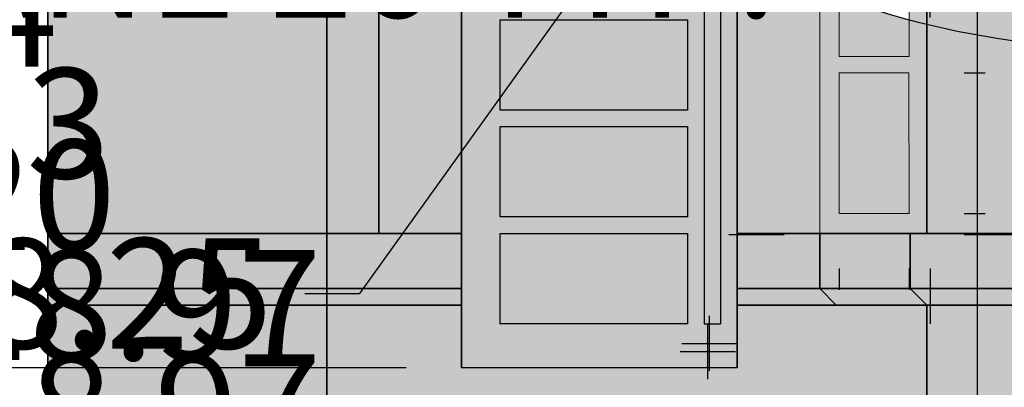
# Model space of a CAD drawing. Units: millimetres. Extents: x 130 to 1021, y 147 to 699.
# Tile 3 of 40: x 302 to 481, y 246 to 313. Entities that reach past the tile are written whole.
import ezdxf

# ---------------------------------------------------------------- set-up
doc = ezdxf.new("R2010")
doc.units = ezdxf.units.MM
doc.header["$MEASUREMENT"] = 0
for name, color, linetype, lineweight in [('A-ANNO-DIMS', 2, 'Continuous', 18), ('A-DOOR', 3, 'Continuous', 25), ('A-ELEV', 7, 'Continuous', 35), ('A-ELEV-PATT', 9, 'Continuous', 13), ('A-FLOR-STRS', 2, 'Continuous', 25), ('A-GLAZ', 4, 'Continuous', 18)]:
    doc.layers.add(name, color=color, linetype=linetype, lineweight=lineweight)
doc.styles.get("Standard").update_dxf_attribs({"font": 'arial.ttf'})
doc.dimstyles.get("Standard").update_dxf_attribs({"dimtxt": 20, "dimasz": 10, "dimexe": 10, "dimexo": 10, "dimgap": 5, "dimtad": 0, "dimtih": 1, "dimtoh": 1, "dimdec": 0, "dimzin": 0, "dimdsep": 46, "dimtxsty": 'Standard', "dimcen": 5, "dimadec": 0, "dimazin": 0, "dimtfac": 1, "dimtdec": 0, "dimtofl": 0, "dimtmove": 0, "dimatfit": 3, "dimfxl": 1, "dimtolj": 1, "dimtzin": 0, "dimarcsym": 0})

# ---------------------------------------------------------------- blocks, each defined once
blk = doc.blocks.new('DOOR-PANEL')
for p, q in [((0, 16.4), (34, 16.4)), ((0, 0), (0, 16.4)), ((34, 16.4), (34, 0)), ((34, 0), (0, 0))]:
    blk.add_line(p, q)
blk = doc.blocks.new('WIN-SIDELIGHT-PANE')
for p, q in [((0, 25.55), (12.68, 25.55)), ((0, 0), (0, 25.55)), ((12.68, 25.55), (12.68, 0)), ((12.68, 0), (0, 0))]:
    blk.add_line(p, q)
blk = doc.blocks.new('*D7')
at = {"layer": 'A-ANNO-DIMS', "color": 0, "lineweight": -2, "transparency": 16777216}
for p, q in [((399.37, 349.45), (413.37, 349.45)), ((423.37, 349.45), (433.37, 349.45)), ((389.37, 344.55), (389.37, 339.45)), ((423.37, 344.55), (423.37, 339.45))]:
    blk.add_line(p, q, dxfattribs=at)
at = {"layer": 'A-ANNO-DIMS', "color": 0, "transparency": 16777216}
for points in [[(399.37, 351.11), (399.37, 347.78), (389.37, 349.45)], [(413.37, 351.11), (413.37, 347.78), (423.37, 349.45)]]:
    blk.add_solid(points, dxfattribs=at)
at = {"layer": 'Defpoints', "color": 0, "transparency": 16777216}
for p in [(389.37, 354.55), (423.37, 354.55), (423.37, 349.45)]:
    blk.add_point(p, dxfattribs=at)
at = {"layer": 'A-ANNO-DIMS', "color": 0, "transparency": 16777216, "insert": (582.04, 349.45), "char_height": 20, "attachment_point": 5}
blk.add_mtext('\\A1;DOOR PANEL 34 TYP.', dxfattribs=at)
blk = doc.blocks.new('*D9')
at = {"layer": 'A-ANNO-DIMS', "color": 0, "lineweight": -2, "transparency": 16777216}
for p, q in [((467.37, 323.13), (457.37, 323.13)), ((467.37, 313.13), (467.37, 323.13)), ((473.55, 303.13), (477.38, 303.13)), ((473.57, 277.58), (477.4, 277.58)), ((467.41, 267.57), (467.42, 257.57))]:
    blk.add_line(p, q, dxfattribs=at)
at = {"layer": 'A-ANNO-DIMS', "color": 0, "transparency": 16777216}
for points in [[(469.04, 313.13), (465.71, 313.13), (467.38, 303.13)], [(469.08, 267.57), (465.75, 267.57), (467.4, 277.57)]]:
    blk.add_solid(points, dxfattribs=at)
at = {"layer": 'Defpoints', "color": 0, "transparency": 16777216}
for p in [(463.55, 303.12), (467.38, 303.13), (463.57, 277.57)]:
    blk.add_point(p, dxfattribs=at)
at = {"layer": 'A-ANNO-DIMS', "color": 0, "transparency": 16777216, "insert": (284.19, 323.13), "char_height": 20, "attachment_point": 5}
blk.add_mtext('\\A1;SIDELIGHT PANE 26 TYP.', dxfattribs=at)
blk = doc.blocks.new('*D10')
at = {"layer": 'A-ANNO-DIMS', "color": 0, "lineweight": -2, "transparency": 16777216}
for p, q in [((440.89, 273.72), (430.89, 273.71)), ((473.57, 273.75), (483.57, 273.75)), ((450.9, 267.56), (450.9, 263.73)), ((463.58, 267.57), (463.58, 263.74))]:
    blk.add_line(p, q, dxfattribs=at)
at = {"layer": 'A-ANNO-DIMS', "color": 0, "transparency": 16777216}
for points in [[(440.89, 275.38), (440.89, 272.05), (450.89, 273.73)], [(473.57, 275.41), (473.58, 272.08), (463.57, 273.74)]]:
    blk.add_solid(points, dxfattribs=at)
at = {"layer": 'Defpoints', "color": 0, "transparency": 16777216}
for p in [(450.89, 277.56), (463.57, 277.57), (463.57, 273.74)]:
    blk.add_point(p, dxfattribs=at)
at = {"layer": 'A-ANNO-DIMS', "color": 0, "transparency": 16777216, "insert": (536.31, 273.75), "char_height": 20, "attachment_point": 5}
blk.add_mtext('\\A1;13 TYP.', dxfattribs=at)
blk = doc.blocks.new('*D11')
at = {"layer": 'A-ANNO-DIMS', "color": 0, "lineweight": -2, "transparency": 16777216}
for p, q in [((737.37, 648.7), (737.37, 149.74)), ((299.37, 566.95), (299.37, 149.74)), ((309.37, 159.74), (490.86, 159.74)), ((727.37, 159.74), (545.89, 159.74))]:
    blk.add_line(p, q, dxfattribs=at)
at = {"layer": 'A-ANNO-DIMS', "color": 0, "transparency": 16777216}
for points in [[(309.37, 161.41), (309.37, 158.07), (299.37, 159.74)], [(727.37, 161.41), (727.37, 158.07), (737.37, 159.74)]]:
    blk.add_solid(points, dxfattribs=at)
at = {"layer": 'Defpoints', "color": 0, "transparency": 16777216}
for p in [(737.37, 658.7), (299.37, 576.95), (737.37, 159.74)]:
    blk.add_point(p, dxfattribs=at)
at = {"layer": 'A-ANNO-DIMS', "color": 0, "transparency": 16777216, "insert": (518.37, 159.74), "char_height": 20, "attachment_point": 5}
blk.add_mtext('\\A1;438', dxfattribs=at)
blk = doc.blocks.new('*D12')
at = {"layer": 'A-ANNO-DIMS', "color": 0, "lineweight": -2, "transparency": 16777216}
for p, q in [((477.37, 661.95), (265.07, 661.95)), ((275.07, 651.95), (275.07, 438.2)), ((275.07, 194.04), (275.07, 407.78)), ((357.16, 184.04), (265.07, 184.04))]:
    blk.add_line(p, q, dxfattribs=at)
at = {"layer": 'A-ANNO-DIMS', "color": 0, "transparency": 16777216}
for points in [[(273.41, 651.95), (276.74, 651.95), (275.07, 661.95)], [(273.41, 194.04), (276.74, 194.04), (275.07, 184.04)]]:
    blk.add_solid(points, dxfattribs=at)
at = {"layer": 'Defpoints', "color": 0, "transparency": 16777216}
for p in [(275.07, 661.95), (487.37, 661.95), (367.16, 184.04)]:
    blk.add_point(p, dxfattribs=at)
at = {"layer": 'A-ANNO-DIMS', "color": 0, "transparency": 16777216, "insert": (275.07, 422.99), "char_height": 20, "attachment_point": 5}
blk.add_mtext('\\A1;477.9', dxfattribs=at)
blk = doc.blocks.new('*D23')
at = {"layer": 'A-ANNO-DIMS', "color": 0, "lineweight": -2, "transparency": 16777216}
for p, q in [((466.77, 403.95), (466.77, 696.25)), ((475.99, 209.04), (475.99, 696.25)), ((456.77, 686.25), (446.77, 686.25)), ((485.99, 686.25), (495.99, 686.25))]:
    blk.add_line(p, q, dxfattribs=at)
at = {"layer": 'A-ANNO-DIMS', "color": 0, "transparency": 16777216}
for points in [[(456.77, 687.91), (456.77, 684.58), (466.77, 686.25)], [(485.99, 687.91), (485.99, 684.58), (475.99, 686.25)]]:
    blk.add_solid(points, dxfattribs=at)
at = {"layer": 'Defpoints', "color": 0, "transparency": 16777216}
for p in [(475.99, 686.25), (466.77, 393.95), (475.99, 199.04)]:
    blk.add_point(p, dxfattribs=at)
at = {"layer": 'A-ANNO-DIMS', "color": 0, "transparency": 16777216, "insert": (534.63, 686.25), "char_height": 20, "attachment_point": 5}
blk.add_mtext('\\A1;9.222', dxfattribs=at)
blk = doc.blocks.new('*D24')
at = {"layer": 'A-ANNO-DIMS', "color": 0, "lineweight": -2, "transparency": 16777216}
for p, q in [((475.99, 209.04), (475.99, 696.25)), ((487.37, 671.95), (487.37, 696.25)), ((465.99, 686.25), (455.99, 686.25)), ((497.37, 686.25), (507.37, 686.25))]:
    blk.add_line(p, q, dxfattribs=at)
at = {"layer": 'A-ANNO-DIMS', "color": 0, "transparency": 16777216}
for points in [[(465.99, 687.91), (465.99, 684.58), (475.99, 686.25)], [(497.37, 687.91), (497.37, 684.58), (487.37, 686.25)]]:
    blk.add_solid(points, dxfattribs=at)
at = {"layer": 'Defpoints', "color": 0, "transparency": 16777216}
for p in [(487.37, 686.25), (487.37, 661.95), (475.99, 199.04)]:
    blk.add_point(p, dxfattribs=at)
at = {"layer": 'A-ANNO-DIMS', "color": 0, "transparency": 16777216, "insert": (553.02, 686.25), "char_height": 20, "attachment_point": 5}
blk.add_mtext('\\A1;11.385', dxfattribs=at)
blk = doc.blocks.new('*D34')
at = {"layer": 'A-ANNO-DIMS', "color": 0, "lineweight": -2, "transparency": 16777216}
for p, q in [((275.07, 231.98), (275.07, 241.98)), ((275.07, 241.98), (285.07, 241.98)), ((459.84, 221.98), (265.07, 221.98)), ((462.91, 203.01), (265.07, 203.01)), ((275.07, 193.01), (275.07, 183.01))]:
    blk.add_line(p, q, dxfattribs=at)
at = {"layer": 'A-ANNO-DIMS', "color": 0, "transparency": 16777216}
for points in [[(273.41, 231.98), (276.74, 231.98), (275.07, 221.98)], [(273.41, 193.01), (276.74, 193.01), (275.07, 203.01)]]:
    blk.add_solid(points, dxfattribs=at)
at = {"layer": 'Defpoints', "color": 0, "transparency": 16777216}
for p in [(275.07, 221.98), (469.84, 221.98), (472.91, 203.01)]:
    blk.add_point(p, dxfattribs=at)
at = {"layer": 'A-ANNO-DIMS', "color": 0, "transparency": 16777216, "insert": (322.88, 241.98), "char_height": 20, "attachment_point": 5}
blk.add_mtext('\\A1;18.97', dxfattribs=at)
blk = doc.blocks.new('*D35')
at = {"layer": 'A-ANNO-DIMS', "color": 0, "lineweight": -2, "transparency": 16777216}
for p, q in [((275.07, 250.95), (275.07, 260.95)), ((275.07, 260.95), (285.07, 260.95)), ((456.77, 240.95), (265.07, 240.95)), ((459.84, 221.98), (265.07, 221.98)), ((275.07, 211.98), (275.07, 201.98))]:
    blk.add_line(p, q, dxfattribs=at)
at = {"layer": 'A-ANNO-DIMS', "color": 0, "transparency": 16777216}
for points in [[(273.41, 250.95), (276.74, 250.95), (275.07, 240.95)], [(273.41, 211.98), (276.74, 211.98), (275.07, 221.98)]]:
    blk.add_solid(points, dxfattribs=at)
at = {"layer": 'Defpoints', "color": 0, "transparency": 16777216}
for p in [(275.07, 240.95), (466.77, 240.95), (469.84, 221.98)]:
    blk.add_point(p, dxfattribs=at)
at = {"layer": 'A-ANNO-DIMS', "color": 0, "transparency": 16777216, "insert": (322.88, 260.95), "char_height": 20, "attachment_point": 5}
blk.add_mtext('\\A1;18.97', dxfattribs=at)
blk = doc.blocks.new('*D36')
at = {"layer": 'A-ANNO-DIMS', "color": 0, "lineweight": -2, "transparency": 16777216}
for p, q in [((275.07, 270.95), (275.07, 280.95)), ((275.07, 280.95), (285.07, 280.95)), ((297.37, 260.95), (265.07, 260.95)), ((456.77, 240.95), (265.07, 240.95)), ((275.07, 230.95), (275.07, 220.95))]:
    blk.add_line(p, q, dxfattribs=at)
at = {"layer": 'A-ANNO-DIMS', "color": 0, "transparency": 16777216}
for points in [[(273.41, 270.95), (276.74, 270.95), (275.07, 260.95)], [(273.41, 230.95), (276.74, 230.95), (275.07, 240.95)]]:
    blk.add_solid(points, dxfattribs=at)
at = {"layer": 'Defpoints', "color": 0, "transparency": 16777216}
for p in [(275.07, 260.95), (307.37, 260.95), (466.77, 240.95)]:
    blk.add_point(p, dxfattribs=at)
at = {"layer": 'A-ANNO-DIMS', "color": 0, "transparency": 16777216, "insert": (304.53, 280.95), "char_height": 20, "attachment_point": 5}
blk.add_mtext('\\A1;20', dxfattribs=at)
blk = doc.blocks.new('*D37')
at = {"layer": 'A-ANNO-DIMS', "color": 0, "lineweight": -2, "transparency": 16777216}
for p, q in [((275.07, 283.95), (275.07, 293.95)), ((275.07, 293.95), (285.07, 293.95)), ((297.37, 273.95), (265.07, 273.95)), ((297.37, 260.95), (265.07, 260.95)), ((275.07, 250.95), (275.07, 240.95))]:
    blk.add_line(p, q, dxfattribs=at)
at = {"layer": 'A-ANNO-DIMS', "color": 0, "transparency": 16777216}
for points in [[(273.41, 283.95), (276.74, 283.95), (275.07, 273.95)], [(273.41, 250.95), (276.74, 250.95), (275.07, 260.95)]]:
    blk.add_solid(points, dxfattribs=at)
at = {"layer": 'Defpoints', "color": 0, "transparency": 16777216}
for p in [(275.07, 273.95), (307.37, 273.95), (307.37, 260.95)]:
    blk.add_point(p, dxfattribs=at)
at = {"layer": 'A-ANNO-DIMS', "color": 0, "transparency": 16777216, "insert": (303.46, 293.95), "char_height": 20, "attachment_point": 5}
blk.add_mtext('\\A1;13', dxfattribs=at)
blk = doc.blocks.new('*D38')
at = {"layer": 'A-ANNO-DIMS', "color": 0, "lineweight": -2, "transparency": 16777216}
for p, q in [((297.37, 388.95), (265.07, 388.95)), ((275.07, 378.95), (275.07, 346.66)), ((275.07, 283.95), (275.07, 316.24)), ((297.37, 273.95), (265.07, 273.95))]:
    blk.add_line(p, q, dxfattribs=at)
at = {"layer": 'A-ANNO-DIMS', "color": 0, "transparency": 16777216}
for points in [[(273.41, 378.95), (276.74, 378.95), (275.07, 388.95)], [(273.41, 283.95), (276.74, 283.95), (275.07, 273.95)]]:
    blk.add_solid(points, dxfattribs=at)
at = {"layer": 'Defpoints', "color": 0, "transparency": 16777216}
for p in [(275.07, 388.95), (307.37, 388.95), (307.37, 273.95)]:
    blk.add_point(p, dxfattribs=at)
at = {"layer": 'A-ANNO-DIMS', "color": 0, "transparency": 16777216, "insert": (275.07, 331.45), "char_height": 20, "attachment_point": 5}
blk.add_mtext('\\A1;115', dxfattribs=at)
blk = doc.blocks.new('*D60')
at = {"layer": 'A-ANNO-DIMS', "color": 0, "lineweight": -2, "transparency": 16777216}
for p, q in [((372.37, 378.95), (265.07, 378.95)), ((275.07, 368.95), (275.07, 329.46)), ((275.07, 259.55), (275.07, 299.04)), ((372.37, 249.55), (265.07, 249.55))]:
    blk.add_line(p, q, dxfattribs=at)
at = {"layer": 'A-ANNO-DIMS', "color": 0, "transparency": 16777216}
for points in [[(273.41, 368.95), (276.74, 368.95), (275.07, 378.95)], [(273.41, 259.55), (276.74, 259.55), (275.07, 249.55)]]:
    blk.add_solid(points, dxfattribs=at)
at = {"layer": 'Defpoints', "color": 0, "transparency": 16777216}
for p in [(275.07, 378.95), (382.37, 378.95), (382.37, 249.55)]:
    blk.add_point(p, dxfattribs=at)
at = {"layer": 'A-ANNO-DIMS', "color": 0, "transparency": 16777216, "insert": (275.07, 314.25), "char_height": 20, "attachment_point": 5}
blk.add_mtext('\\A1;129.4', dxfattribs=at)
blk = doc.blocks.new('*D64')
at = {"layer": 'A-ANNO-DIMS', "color": 0, "lineweight": -2, "transparency": 16777216}
for p, q in [((502.05, 450.93), (502.05, 460.93)), ((497.05, 455.93), (507.05, 455.93)), ((363.96, 263.06), (409.92, 327.25)), ((353.96, 263.06), (363.96, 263.06))]:
    blk.add_line(p, q, dxfattribs=at)
at = {"layer": 'A-ANNO-DIMS', "color": 0, "transparency": 16777216}
blk.add_solid([(408.57, 328.22), (411.28, 326.28), (415.74, 335.39)], dxfattribs=at)
at = {"layer": 'Defpoints', "color": 0, "transparency": 16777216}
for p in [(502.05, 455.93), (415.74, 335.39)]:
    blk.add_point(p, dxfattribs=at)
at = {"layer": 'A-ANNO-DIMS', "color": 0, "transparency": 16777216, "insert": (297.8, 263.06), "char_height": 20, "attachment_point": 5}
blk.add_mtext('\\A1;R148.25', dxfattribs=at)
blk = doc.blocks.new('*D65')
at = {"layer": 'A-ANNO-DIMS', "color": 0, "lineweight": -2, "transparency": 16777216}
for p, q in [((495.46, 509.13), (472.51, 423.11)), ((505.46, 509.13), (495.46, 509.13)), ((427.37, 248.98), (427.37, 258.98)), ((422.37, 253.98), (432.37, 253.98))]:
    blk.add_line(p, q, dxfattribs=at)
at = {"layer": 'A-ANNO-DIMS', "color": 0, "transparency": 16777216}
blk.add_solid([(470.9, 423.54), (474.12, 422.68), (469.93, 413.45)], dxfattribs=at)
at = {"layer": 'Defpoints', "color": 0, "transparency": 16777216}
for p in [(469.93, 413.45), (427.37, 253.98)]:
    blk.add_point(p, dxfattribs=at)
at = {"layer": 'A-ANNO-DIMS', "color": 0, "transparency": 16777216, "insert": (561.62, 509.13), "char_height": 20, "attachment_point": 5}
blk.add_mtext('\\A1;R165.05', dxfattribs=at)
blk = doc.blocks.new('*D67')
at = {"layer": 'A-ANNO-DIMS', "color": 0, "lineweight": -2, "transparency": 16777216}
for p, q in [((479.76, 492.43), (462.14, 412.22)), ((489.76, 492.43), (479.76, 492.43)), ((427.07, 247.5), (427.07, 257.5)), ((422.07, 252.5), (432.07, 252.5))]:
    blk.add_line(p, q, dxfattribs=at)
at = {"layer": 'A-ANNO-DIMS', "color": 0, "transparency": 16777216}
blk.add_solid([(460.52, 412.58), (463.77, 411.87), (460, 402.46)], dxfattribs=at)
at = {"layer": 'Defpoints', "color": 0, "transparency": 16777216}
for p in [(460, 402.46), (427.07, 252.5)]:
    blk.add_point(p, dxfattribs=at)
at = {"layer": 'A-ANNO-DIMS', "color": 0, "transparency": 16777216, "insert": (545.84, 492.43), "char_height": 20, "attachment_point": 5}
blk.add_mtext('\\A1;R153.53', dxfattribs=at)

msp = doc.modelspace()

# ---------------------------------------------------------------- hatches: boundary and pattern name
at = {"layer": 'A-ELEV-PATT'}
h = msp.add_hatch(color=256, dxfattribs=at)
h.dxf.hatch_style = 1
h.paths.add_polyline_path([(737.3738, 658.6988, 0.01359606), (632.4019, 661.9473), (607.3738, 661.9473), (487.3738, 661.9473), (487.3738, 649.9473), (607.3738, 649.9473), (632.3794, 649.9473, -0.01368411), (737.3738, 646.6784)])
h.paths.add_polyline_path([(732.3738, 643.9599, 0.01305286), (632.3738, 646.9473), (607.3738, 646.9473), (487.3738, 646.9473), (487.3738, 596.9473), (632.3738, 596.9473, -0.01305286), (732.3738, 593.9599)])
h.paths.add_polyline_path([(737.3738, 593.6732, 0.01370629), (632.3738, 596.9473), (487.3738, 596.9473), (487.3738, 586.9473), (632.355, 586.9473, -0.01378075), (737.3738, 583.6559)])
h.paths.add_polyline_path([(447.3738, 646.9473), (307.3738, 646.9473), (302.3738, 646.9473), (302.3738, 634.9473), (447.3738, 634.9473)])
h.paths.add_polyline_path([(447.3738, 631.9473), (307.3738, 631.9473), (307.3738, 586.9473), (447.3738, 586.9473)])
h.paths.add_polyline_path([(447.3738, 586.9473), (307.3738, 586.9473), (302.3738, 586.9473), (302.3738, 576.9473), (447.3738, 576.9473)])
h.paths.add_polyline_path([(447.3738, 573.9473), (367.3738, 573.9473), (367.3738, 539.9473), (447.3738, 539.9473)])
h.paths.add_polyline_path([(447.3738, 537.9473), (367.3738, 537.9473), (367.3738, 507.9473), (400.392, 507.4253, -0.00172798), (401.3281, 507.6451, -0.52200255), (425.6117, 511.0391, -0.03918489), (447.3738, 510.4359), (447.3738, 510.7883)])
h.paths.add_polyline_path([(394.7238, 505.9473), (367.3738, 505.9473), (367.3738, 476.9473, -0.0146512), (375.8501, 480.2159), (376.1506, 499.2266, -0.03554194)])
h.paths.add_polyline_path([(632.3738, 583.9473), (552.3738, 583.9473), (552.3738, 550.9473), (632.3738, 550.9473)])
h.paths.add_polyline_path([(632.3738, 548.9473), (552.3738, 548.9473), (552.3738, 515.9473), (632.3738, 515.9473)])
h.paths.add_polyline_path([(632.3738, 513.9473), (552.3738, 513.9473), (552.3738, 476.9473), (632.3738, 476.9473)])
h.paths.add_polyline_path([(737.3738, 473.6903, 0.01363261), (632.3926, 476.9473), (552.3738, 476.9473), (487.3738, 476.9473), (487.3738, 466.9473), (632.3738, 466.9473, -0.01370629), (737.3738, 463.6732)])
h.paths.add_polyline_path([(732.3738, 460.9552, 0.01307409), (632.3681, 463.9473), (487.3738, 463.9473), (487.3738, 407.735, -0.00322862), (489.3544, 406.9473), (632.3926, 406.9473, -0.01298259), (732.3738, 403.9755)])
h.paths.add_polyline_path([(487.3738, 463.9473, 0.20132998), (367.3738, 463.9473), (367.3738, 407.735, -0.18820307), (487.3738, 407.735)])
h.paths.add_polyline_path([(367.3738, 476.9473), (367.3738, 466.9473, -0.20133085), (487.3738, 466.9473), (487.3738, 476.9473, 0.20132998)])
h.paths.add_polyline_path([(367.3738, 463.9473), (307.3738, 463.9473), (307.3738, 401.9473), (357.9413, 401.9473), (367.3738, 407.735)])
h.paths.add_polyline_path([(367.3738, 476.9473), (302.3738, 476.9473), (302.3738, 466.9473), (367.3738, 466.9473)])
h.paths.add_polyline_path([(632.8184, 366.9453), (552.3738, 366.9453), (552.3738, 393.9473), (632.8184, 393.9473)])
h.paths.add_polyline_path([(632.8184, 357.2114), (632.8184, 363.9453), (552.3738, 363.9453), (552.3738, 357.2114), (552.3738, 336.9453), (632.8184, 336.9453)])
h.paths.add_polyline_path([(632.8184, 333.9453), (552.3738, 333.9453), (552.3738, 306.9453), (632.8184, 306.9453)])
h.paths.add_polyline_path([(632.8184, 303.9453), (552.3738, 303.9453), (552.3738, 273.9473), (632.355, 273.9473, 0.00006077), (632.8184, 273.9491)])
h.paths.add_polyline_path([(737.3738, 403.6903, 0.01363261), (632.3926, 406.9473), (489.3544, 406.9473, 0.19154808), (367.3738, 407.735), (367.3738, 396.9473, -0.20133085), (487.3738, 396.9473), (632.3738, 396.9473, -0.01370629), (737.3738, 393.6732)])
h.paths.add_polyline_path([(357.9413, 401.9473), (307.3738, 401.9473), (307.3738, 391.9473), (357.9413, 391.9473)])
h.paths.add_polyline_path([(357.9413, 357.2114), (357.9413, 388.9473), (307.3738, 388.9473), (307.3738, 357.2114), (307.3738, 273.9473), (357.9413, 273.9473)])
h.paths.add_polyline_path([(732.3738, 263.93, -0.0130317), (632.3794, 260.9473), (466.7667, 260.9473), (466.7667, 240.9473), (469.8406, 236.978), (469.8406, 221.978), (472.9145, 218.0087), (472.9145, 213.9473), (607.3738, 213.9473), (732.3738, 213.9473)])
h.paths.add_polyline_path([(732.3738, 290.889), (722.479, 290.889), (722.479, 301.889), (732.3738, 301.889), (732.3738, 305.889), (722.479, 305.889), (722.479, 316.889), (732.3738, 316.889), (732.3738, 320.889), (722.479, 320.889), (722.479, 331.889), (732.3738, 331.889), (732.3738, 335.889), (722.479, 335.889), (722.479, 346.889), (732.3738, 346.889), (732.3738, 350.889), (722.479, 350.889), (722.479, 361.889), (732.3738, 361.889), (732.3738, 365.889), (722.479, 365.889), (722.479, 376.889), (732.3738, 376.889), (732.3738, 380.889), (722.479, 380.889), (722.479, 391.4848, 0.00052326), (718.479, 391.6843), (718.479, 380.889), (707.479, 380.889), (707.479, 392.1896, 0.00052307), (703.479, 392.3576), (703.479, 380.889), (692.479, 380.889), (692.479, 392.7765, 0.00052292), (688.479, 392.9131), (688.479, 380.889), (677.479, 380.889), (677.479, 393.2456, 0.00052279), (673.479, 393.3508), (673.479, 380.889), (662.479, 380.889), (662.479, 393.597, 0.0005227), (658.479, 393.6709), (658.479, 380.889), (647.479, 380.889), (647.479, 393.8308, 0.00052264), (643.479, 393.8732), (643.479, 380.889), (632.8184, 380.889), (632.8184, 376.889), (643.479, 376.889), (643.479, 365.889), (632.8184, 365.889), (632.8184, 361.889), (643.479, 361.889), (643.479, 350.889), (632.8184, 350.889), (632.8184, 346.889), (643.479, 346.889), (643.479, 335.889), (632.8184, 335.889), (632.8184, 331.889), (643.479, 331.889), (643.479, 320.889), (632.8184, 320.889), (632.8184, 316.889), (643.479, 316.889), (643.479, 305.889), (632.8184, 305.889), (632.8184, 301.889), (643.479, 301.889), (643.479, 290.889), (632.8184, 290.889), (632.8184, 286.889), (643.479, 286.889), (643.479, 274.0217, 0.00052456), (647.479, 274.0643), (647.479, 286.889), (658.479, 286.889), (658.479, 274.2248, 0.00052462), (662.479, 274.2989), (662.479, 286.889), (673.479, 286.889), (673.479, 274.546, 0.00052471), (677.479, 274.6516), (677.479, 286.889), (688.479, 286.889), (688.479, 274.9853, 0.00052484), (692.479, 275.1224), (692.479, 286.889), (703.479, 286.889), (703.479, 275.5429, 0.000525), (707.479, 275.7115), (707.479, 286.889), (718.479, 286.889), (718.479, 276.2187, 0.00052519), (722.479, 276.4189), (722.479, 286.889), (732.3738, 286.889)])
h.paths.add_polyline_path([(718.479, 290.889), (707.479, 290.889), (707.479, 301.889), (718.479, 301.889)], flags=16)
h.paths.add_polyline_path([(703.479, 290.889), (692.479, 290.889), (692.479, 301.889), (703.479, 301.889)], flags=16)
h.paths.add_polyline_path([(718.479, 305.889), (707.479, 305.889), (707.479, 316.889), (718.479, 316.889)], flags=16)
h.paths.add_polyline_path([(703.479, 305.889), (692.479, 305.889), (692.479, 316.889), (703.479, 316.889)], flags=16)
h.paths.add_polyline_path([(688.479, 290.889), (677.479, 290.889), (677.479, 301.889), (688.479, 301.889)], flags=16)
h.paths.add_polyline_path([(718.479, 320.889), (707.479, 320.889), (707.479, 331.889), (718.479, 331.889)], flags=16)
h.paths.add_polyline_path([(688.479, 305.889), (677.479, 305.889), (677.479, 316.889), (688.479, 316.889)], flags=16)
h.paths.add_polyline_path([(703.479, 320.889), (692.479, 320.889), (692.479, 331.889), (703.479, 331.889)], flags=16)
h.paths.add_polyline_path([(688.479, 320.889), (677.479, 320.889), (677.479, 331.889), (688.479, 331.889)], flags=16)
h.paths.add_polyline_path([(673.479, 290.889), (662.479, 290.889), (662.479, 301.889), (673.479, 301.889)], flags=16)
h.paths.add_polyline_path([(718.479, 335.889), (707.479, 335.889), (707.479, 346.889), (718.479, 346.889)], flags=16)
h.paths.add_polyline_path([(673.479, 305.889), (662.479, 305.889), (662.479, 316.889), (673.479, 316.889)], flags=16)
h.paths.add_polyline_path([(703.479, 335.889), (692.479, 335.889), (692.479, 346.889), (703.479, 346.889)], flags=16)
h.paths.add_polyline_path([(673.479, 320.889), (662.479, 320.889), (662.479, 331.889), (673.479, 331.889)], flags=16)
h.paths.add_polyline_path([(688.479, 335.889), (677.479, 335.889), (677.479, 346.889), (688.479, 346.889)], flags=16)
h.paths.add_polyline_path([(658.479, 290.889), (647.479, 290.889), (647.479, 301.889), (658.479, 301.889)], flags=16)
h.paths.add_polyline_path([(718.479, 350.889), (707.479, 350.889), (707.479, 361.889), (718.479, 361.889)], flags=16)
h.paths.add_polyline_path([(658.479, 305.889), (647.479, 305.889), (647.479, 316.889), (658.479, 316.889)], flags=16)
h.paths.add_polyline_path([(703.479, 350.889), (692.479, 350.889), (692.479, 361.889), (703.479, 361.889)], flags=16)
h.paths.add_polyline_path([(673.479, 335.889), (662.479, 335.889), (662.479, 346.889), (673.479, 346.889)], flags=16)
h.paths.add_polyline_path([(658.479, 320.889), (647.479, 320.889), (647.479, 331.889), (658.479, 331.889)], flags=16)
h.paths.add_polyline_path([(688.479, 350.889), (677.479, 350.889), (677.479, 361.889), (688.479, 361.889)], flags=16)
h.paths.add_polyline_path([(718.479, 365.889), (707.479, 365.889), (707.479, 376.889), (718.479, 376.889)], flags=16)
h.paths.add_polyline_path([(658.479, 335.889), (647.479, 335.889), (647.479, 346.889), (658.479, 346.889)], flags=16)
h.paths.add_polyline_path([(673.479, 350.889), (662.479, 350.889), (662.479, 361.889), (673.479, 361.889)], flags=16)
h.paths.add_polyline_path([(703.479, 365.889), (692.479, 365.889), (692.479, 376.889), (703.479, 376.889)], flags=16)
h.paths.add_polyline_path([(688.479, 365.889), (677.479, 365.889), (677.479, 376.889), (688.479, 376.889)], flags=16)
h.paths.add_polyline_path([(658.479, 350.889), (647.479, 350.889), (647.479, 361.889), (658.479, 361.889)], flags=16)
h.paths.add_polyline_path([(673.479, 365.889), (662.479, 365.889), (662.479, 376.889), (673.479, 376.889)], flags=16)
h.paths.add_polyline_path([(658.479, 365.889), (647.479, 365.889), (647.479, 376.889), (658.479, 376.889)], flags=16)
h.paths.add_polyline_path([(732.3738, 503.9786), (722.3392, 503.9786), (722.3392, 514.9786), (732.3738, 514.9786), (732.3738, 518.9786), (722.3392, 518.9786), (722.3392, 529.9786), (732.3738, 529.9786), (732.3738, 533.9786), (722.3392, 533.9786), (722.3392, 544.9786), (732.3738, 544.9786), (732.3738, 546.9473), (732.3738, 548.9786), (722.3392, 548.9786), (722.3392, 559.9786), (732.3738, 559.9786), (732.3738, 563.9786), (722.3392, 563.9786), (722.3392, 574.9786), (732.3738, 574.9786), (732.3738, 578.9786), (722.3392, 578.9786), (722.3392, 581.4789, 0.00052601), (718.3392, 581.6791), (718.3392, 578.9786), (707.3392, 578.9786), (707.3392, 582.1863, 0.00052582), (703.3392, 582.355), (703.3392, 578.9786), (692.3392, 578.9786), (692.3392, 582.7752, 0.00052566), (688.3392, 582.9123), (688.3392, 578.9786), (677.3392, 578.9786), (677.3392, 583.2457, 0.00052554), (673.3392, 583.3512), (673.3392, 578.9786), (662.3392, 578.9786), (662.3392, 583.5978, 0.00052545), (658.3392, 583.6718), (658.3392, 578.9786), (647.3392, 578.9786), (647.3392, 583.8317, 0.00052539), (643.3392, 583.8741), (643.3392, 578.9786), (632.3738, 578.9786), (632.3738, 574.9786), (643.3392, 574.9786), (643.3392, 563.9786), (632.3738, 563.9786), (632.3738, 559.9786), (643.3392, 559.9786), (643.3392, 548.9786), (632.3738, 548.9786), (632.3738, 544.9786), (643.3392, 544.9786), (643.3392, 533.9786), (632.3738, 533.9786), (632.3738, 529.9786), (643.3392, 529.9786), (643.3392, 518.9786), (632.3738, 518.9786), (632.3738, 515.9473), (632.3738, 514.9786), (643.3392, 514.9786), (643.3392, 503.9786), (632.3738, 503.9786), (632.3738, 499.9786), (643.3392, 499.9786), (643.3392, 488.9786), (632.3738, 488.9786), (632.3738, 484.9786), (643.3392, 484.9786), (643.3392, 476.8751, -0.00051911), (647.3392, 476.8332), (647.3392, 484.9786), (658.3392, 484.9786), (658.3392, 476.6752, -0.00051917), (662.3392, 476.6022), (662.3392, 484.9786), (673.3392, 484.9786), (673.3392, 476.3585, -0.00051926), (677.3392, 476.2543), (677.3392, 484.9786), (688.3392, 484.9786), (688.3392, 475.9248, -0.00051938), (692.3392, 475.7894), (692.3392, 484.9786), (703.3392, 484.9786), (703.3392, 475.3741, -0.00051953), (707.3392, 475.2075), (707.3392, 484.9786), (718.3392, 484.9786), (718.3392, 474.7064, -0.00051972), (722.3392, 474.5086), (722.3392, 484.9786), (732.3738, 484.9786), (732.3738, 488.9786), (722.3392, 488.9786), (722.3392, 499.9786), (732.3738, 499.9786)])
h.paths.add_polyline_path([(718.3392, 503.9786), (707.3392, 503.9786), (707.3392, 514.9786), (718.3392, 514.9786)], flags=16)
h.paths.add_polyline_path([(718.3392, 499.9786), (718.3392, 488.9786), (707.3392, 488.9786), (707.3392, 499.9786)], flags=16)
h.paths.add_polyline_path([(718.3392, 518.9786), (707.3392, 518.9786), (707.3392, 529.9786), (718.3392, 529.9786)], flags=16)
h.paths.add_polyline_path([(703.3392, 503.9786), (692.3392, 503.9786), (692.3392, 514.9786), (703.3392, 514.9786)], flags=16)
h.paths.add_polyline_path([(703.3392, 499.9786), (703.3392, 488.9786), (692.3392, 488.9786), (692.3392, 499.9786)], flags=16)
h.paths.add_polyline_path([(703.3392, 518.9786), (692.3392, 518.9786), (692.3392, 529.9786), (703.3392, 529.9786)], flags=16)
h.paths.add_polyline_path([(718.3392, 533.9786), (707.3392, 533.9786), (707.3392, 544.9786), (718.3392, 544.9786)], flags=16)
h.paths.add_polyline_path([(688.3392, 503.9786), (677.3392, 503.9786), (677.3392, 514.9786), (688.3392, 514.9786)], flags=16)
h.paths.add_polyline_path([(688.3392, 499.9786), (688.3392, 488.9786), (677.3392, 488.9786), (677.3392, 499.9786)], flags=16)
h.paths.add_polyline_path([(703.3392, 533.9786), (692.3392, 533.9786), (692.3392, 544.9786), (703.3392, 544.9786)], flags=16)
h.paths.add_polyline_path([(688.3392, 518.9786), (677.3392, 518.9786), (677.3392, 529.9786), (688.3392, 529.9786)], flags=16)
h.paths.add_polyline_path([(688.3392, 533.9786), (677.3392, 533.9786), (677.3392, 544.9786), (688.3392, 544.9786)], flags=16)
h.paths.add_polyline_path([(718.3392, 548.9786), (707.3392, 548.9786), (707.3392, 559.9786), (718.3392, 559.9786)], flags=16)
h.paths.add_polyline_path([(673.3392, 503.9786), (662.3392, 503.9786), (662.3392, 514.9786), (673.3392, 514.9786)], flags=16)
h.paths.add_polyline_path([(673.3392, 499.9786), (673.3392, 488.9786), (662.3392, 488.9786), (662.3392, 499.9786)], flags=16)
h.paths.add_polyline_path([(703.3392, 548.9786), (692.3392, 548.9786), (692.3392, 559.9786), (703.3392, 559.9786)], flags=16)
h.paths.add_polyline_path([(673.3392, 518.9786), (662.3392, 518.9786), (662.3392, 529.9786), (673.3392, 529.9786)], flags=16)
h.paths.add_polyline_path([(688.3392, 548.9786), (677.3392, 548.9786), (677.3392, 559.9786), (688.3392, 559.9786)], flags=16)
h.paths.add_polyline_path([(673.3392, 533.9786), (662.3392, 533.9786), (662.3392, 544.9786), (673.3392, 544.9786)], flags=16)
h.paths.add_polyline_path([(718.3392, 563.9786), (707.3392, 563.9786), (707.3392, 574.9786), (718.3392, 574.9786)], flags=16)
h.paths.add_polyline_path([(658.3392, 503.9786), (647.3392, 503.9786), (647.3392, 514.9786), (658.3392, 514.9786)], flags=16)
h.paths.add_polyline_path([(658.3392, 499.9786), (658.3392, 488.9786), (647.3392, 488.9786), (647.3392, 499.9786)], flags=16)
h.paths.add_polyline_path([(703.3392, 563.9786), (692.3392, 563.9786), (692.3392, 574.9786), (703.3392, 574.9786)], flags=16)
h.paths.add_polyline_path([(658.3392, 518.9786), (647.3392, 518.9786), (647.3392, 529.9786), (658.3392, 529.9786)], flags=16)
h.paths.add_polyline_path([(673.3392, 548.9786), (662.3392, 548.9786), (662.3392, 559.9786), (673.3392, 559.9786)], flags=16)
h.paths.add_polyline_path([(688.3392, 563.9786), (677.3392, 563.9786), (677.3392, 574.9786), (688.3392, 574.9786)], flags=16)
h.paths.add_polyline_path([(658.3392, 533.9786), (647.3392, 533.9786), (647.3392, 544.9786), (658.3392, 544.9786)], flags=16)
h.paths.add_polyline_path([(673.3392, 563.9786), (662.3392, 563.9786), (662.3392, 574.9786), (673.3392, 574.9786)], flags=16)
h.paths.add_polyline_path([(658.3392, 548.9786), (647.3392, 548.9786), (647.3392, 559.9786), (658.3392, 559.9786)], flags=16)
h.paths.add_polyline_path([(658.3392, 563.9786), (647.3392, 563.9786), (647.3392, 574.9786), (658.3392, 574.9786)], flags=16)
h = msp.add_hatch(color=256, dxfattribs=at)
h.dxf.hatch_style = 1
h.paths.add_polyline_path([(447.3738, 576.9473), (302.3738, 576.9473), (302.3738, 573.9473), (447.3738, 573.9473)])
h.paths.add_polyline_path([(487.3738, 583.9473), (487.3738, 586.9473), (447.3738, 576.9473), (447.3738, 573.9473)])
h.paths.add_polyline_path([(632.355, 586.9473), (487.3738, 586.9473), (487.3738, 583.9473), (632.3738, 583.9473), (632.3738, 583.9472, -0.01380003), (737.3738, 580.6507), (737.3738, 583.6559, 0.01378075)])
h.paths.add_polyline_path([(367.3738, 466.9473), (302.3738, 466.9473), (302.3738, 463.9473), (367.3738, 463.9473)])
h.paths.add_polyline_path([(487.3738, 463.9473), (487.3738, 466.9473, 0.20133085), (367.3738, 466.9473), (367.3738, 463.9473, -0.20132998)])
h.paths.add_polyline_path([(632.3738, 466.9473), (487.3738, 466.9473), (487.3738, 463.9473), (632.3681, 463.9473, -0.01372855), (737.3738, 460.6681), (737.3738, 463.6732, 0.01370629)])
h.paths.add_polyline_path([(632.3738, 396.9473), (487.3738, 396.9473, 0.20133085), (367.3738, 396.9473), (367.3738, 393.9473, -0.20237172), (486.7667, 393.9473), (632.3681, 393.9473, -0.01372855), (737.3738, 390.6681), (737.3738, 393.6732, 0.01370629)])
h.paths.add_polyline_path([(357.9413, 391.9473), (307.3738, 391.9473), (307.3738, 388.9473), (357.9413, 388.9473)])
h.paths.add_polyline_path([(367.3738, 393.9473), (367.3738, 396.9473), (357.9413, 391.924), (357.9413, 388.9473), (358.058, 388.9473)])
h.paths.add_polyline_path([(737.3738, 264.2162), (737.3738, 267.2214, -0.01370629), (632.3738, 263.9473), (463.7667, 263.9473), (466.7667, 260.9473), (632.3794, 260.9473, 0.01368411)])
h.paths.add_polyline_path([(463.7667, 263.9473), (447.3738, 263.9473), (450.3738, 260.9473), (466.7667, 260.9473)])
h.paths.add_polyline_path([(447.3738, 263.9473), (432.3738, 263.9473), (432.3738, 260.9473), (450.3738, 260.9473)])
h.paths.add_polyline_path([(382.3738, 263.9473), (357.9413, 263.9473), (357.9413, 260.9473), (382.3738, 260.9473)])
h.paths.add_polyline_path([(357.9413, 263.9473), (307.3738, 263.9473), (307.3738, 260.9473), (357.9413, 260.9473)])
h = msp.add_hatch(color=256, dxfattribs=at)
h.paths.add_polyline_path([(327.3738, 569.884), (327.3738, 573.9473), (307.3738, 573.9473), (307.3738, 476.9473), (327.3738, 476.9473), (327.3738, 480.95)])
h.paths.add_polyline_path([(486.7667, 386.2639), (486.7667, 393.9473), (466.7667, 393.9473), (466.7667, 357.2114), (466.7667, 311.9335, 0.03427026), (486.7667, 308.4637)])
h.paths.add_polyline_path([(486.7667, 308.4637, -0.03427026), (466.7667, 311.9335), (466.7667, 273.9473), (486.7667, 273.9473)])
h.paths.add_polyline_path([(389.3738, 351.5473), (396.7693, 351.5473, -0.00702703), (393.8774, 354.5473), (389.3738, 354.5473), (389.3738, 359.5775, -0.01903024), (382.3738, 368.424), (382.3738, 249.5473), (432.3738, 249.5473), (432.3738, 325.067, -0.00576734), (429.3738, 326.709), (429.3738, 257.5473), (426.3738, 257.5473), (426.3738, 328.4428, -0.00592542), (423.3738, 330.272), (423.3738, 315.7473), (389.3738, 315.7473), (389.3738, 332.1473), (420.4552, 332.1473, -0.00895099), (416.0768, 335.1473), (389.3738, 335.1473)])
h.paths.add_polyline_path([(389.3738, 312.7473), (423.3738, 312.7473), (423.3738, 296.3473), (389.3738, 296.3473)], flags=16)
h.paths.add_polyline_path([(389.3738, 293.3473), (423.3738, 293.3473), (423.3738, 276.9473), (389.3738, 276.9473)], flags=16)
h.paths.add_polyline_path([(389.3738, 273.9473), (423.3738, 273.9473), (423.3738, 257.5473), (389.3738, 257.5473)], flags=16)
h.paths.add_polyline_path([(432.3738, 378.9473), (382.3738, 378.9473), (382.3738, 368.424, 0.01903024), (389.3738, 359.5775), (389.3738, 370.9473), (423.3738, 370.9473), (423.3738, 354.5473), (393.8774, 354.5473, 0.00702703), (396.7693, 351.5473), (423.3738, 351.5473), (423.3738, 335.1473), (416.0768, 335.1473, 0.00895099), (420.4552, 332.1473), (423.3738, 332.1473), (423.3738, 330.272, 0.00592542), (426.3738, 328.4428), (426.3738, 370.9473), (429.3738, 370.9473), (429.3738, 326.709, 0.00576734), (432.3738, 325.067)])
h.paths.add_polyline_path([(466.7667, 357.2114), (466.7667, 393.9473), (447.3738, 393.9473), (447.3738, 357.2114), (447.3738, 318.1243, 0.0063261), (450.8779, 316.785), (450.8779, 331.5915), (463.5608, 331.5915), (463.5608, 312.7571, 0.00558197), (466.7667, 311.9335)])
h.paths.add_polyline_path([(450.8779, 334.5915), (450.8779, 360.0915), (463.5608, 360.0915), (463.5608, 334.5915)], flags=16)
h.paths.add_polyline_path([(450.8779, 363.0915), (450.8779, 388.6449), (463.5608, 388.6449), (463.5608, 363.0915)], flags=16)
h.paths.add_polyline_path([(466.7667, 311.9335, -0.00558197), (463.5608, 312.7571), (463.5608, 306.0915), (450.8779, 306.0915), (450.8779, 316.785, -0.0063261), (447.3738, 318.1243), (447.3738, 273.9473), (466.7667, 273.9473)])
h.paths.add_polyline_path([(450.8779, 303.0915), (463.5608, 303.0915), (463.5608, 277.5915), (450.8779, 277.5915)], flags=16)
h.paths.add_polyline_path([(552.3738, 357.2114), (552.3738, 393.9473), (486.7667, 393.9473), (486.7667, 386.2639), (544.6354, 386.2639), (544.6354, 280.6619), (486.7667, 280.6619), (486.7667, 273.9473), (552.3738, 273.9473)])
h.paths.add_polyline_path([(487.3738, 583.9473), (472.3738, 580.1973), (472.3738, 507.0765), (472.3738, 505.4251, -0.00564525), (475.3738, 504.4942), (475.3738, 506.3543), (475.3738, 511.9473), (484.3738, 511.9473), (484.3738, 503.8134), (484.3738, 501.2439, -0.00583574), (487.3738, 500.0015)])
h.paths.add_polyline_path([(484.3738, 578.0434), (484.3738, 548.9473), (475.3738, 548.9473), (475.3738, 575.7934)], flags=16)
h.paths.add_polyline_path([(484.3738, 546.9473), (484.3738, 513.9473), (475.3738, 513.9473), (475.3738, 518.7148), (475.3738, 546.9473)], flags=16)
h = msp.add_hatch(color=256, dxfattribs=at)
h.dxf.hatch_style = 1
h.paths.add_polyline_path([(367.3738, 407.735), (357.9413, 401.9473), (357.9413, 391.9473), (357.985, 391.9473), (367.3738, 396.9473)])
h.paths.add_polyline_path([(367.3738, 393.9473), (357.9413, 388.8847), (357.9413, 357.2114), (357.9413, 273.9473), (367.3738, 273.9473), (367.3738, 357.2114)])
h = msp.add_hatch(color=256, dxfattribs=at)
h.dxf.hatch_style = 1
h.paths.add_polyline_path([(382.3738, 368.424, -0.05004781), (367.3738, 393.9473), (367.3738, 357.2114), (367.3738, 273.9473), (382.3738, 273.9473)])
h.paths.add_polyline_path([(432.3738, 273.9473), (447.3738, 273.9473), (447.3738, 318.1243, -0.02789446), (432.3738, 325.067)])
h.paths.add_polyline_path([(463.5608, 306.0915), (463.5608, 312.7571, -0.02245133), (450.8779, 316.785), (450.8779, 306.0915)])
h.paths.add_polyline_path([(450.8779, 303.0915), (450.8779, 277.5915), (463.5608, 277.5915), (463.5608, 303.0915)])
h = msp.add_hatch(color=256, dxfattribs=at)
h.set_gradient(color1=(221, 197, 207), color2=(86, 84, 89), name='CURVED')
h.paths.add_polyline_path([(423.3738, 273.9473), (389.3738, 273.9473), (389.3738, 257.5473), (423.3738, 257.5473)])
h.paths.add_polyline_path([(423.3738, 293.3473), (389.3738, 293.3473), (389.3738, 276.9473), (423.3738, 276.9473)])
h.paths.add_polyline_path([(423.3738, 312.7473), (389.3738, 312.7473), (389.3738, 296.3473), (423.3738, 296.3473)])
h.paths.add_polyline_path([(423.3738, 330.272, -0.00585023), (420.4552, 332.1473), (389.3738, 332.1473), (389.3738, 315.7473), (423.3738, 315.7473)])
h.paths.add_polyline_path([(396.7693, 351.5473), (389.3738, 351.5473), (389.3738, 335.1473), (416.0768, 335.1473, -0.04279691)])
h.paths.add_polyline_path([(423.3738, 351.5473), (396.7693, 351.5473, 0.04279691), (416.0768, 335.1473), (423.3738, 335.1473)])
h.paths.add_polyline_path([(423.3738, 370.9473), (389.3738, 370.9473), (389.3738, 359.5775, 0.01138691), (393.8774, 354.5473), (423.3738, 354.5473)])
h.paths.add_polyline_path([(389.3738, 359.5775), (389.3738, 354.5473), (393.8774, 354.5473, -0.01138691)], flags=17)
h = msp.add_hatch(color=256, dxfattribs=at)
h.set_gradient(color1=(221, 197, 207), color2=(86, 84, 89), name='CURVED')
h.paths.add_polyline_path([(429.3738, 326.709, -0.00584318), (426.3738, 328.4428), (426.3738, 257.5473), (429.3738, 257.5473)])
h.paths.add_polyline_path([(426.3738, 328.4428, 0.00584318), (429.3738, 326.709), (429.3738, 370.9473), (426.3738, 370.9473)])
h = msp.add_hatch(color=256, dxfattribs=at)
h.dxf.hatch_style = 1
h.paths.add_polyline_path([(463.7667, 273.9473), (463.7667, 263.9473), (632.3738, 263.9473, 0.01370629), (737.3738, 267.2214), (737.3738, 277.2387, -0.01378075), (632.355, 273.9473)])
h = msp.add_hatch(color=256, dxfattribs=at)
h.dxf.hatch_style = 1
h.paths.add_polyline_path([(357.9413, 240.9473), (357.9413, 260.9473), (307.3738, 260.9473), (307.3738, 213.9473), (357.9413, 213.9473)])
h.paths.add_polyline_path([(382.3738, 260.9473), (357.9413, 260.9473), (357.9413, 240.9473), (466.7667, 240.9473), (466.7667, 260.9473), (432.3738, 260.9473), (432.3738, 249.5473), (382.3738, 249.5473)])
h.paths.add_polyline_path([(357.9413, 273.9473), (307.3738, 273.9473), (307.3738, 263.9473), (357.9413, 263.9473)])
h.paths.add_polyline_path([(382.3738, 273.9473), (357.9413, 273.9473), (357.9413, 263.9473), (382.3738, 263.9473)])
msp.add_hatch(color=256, dxfattribs=at).paths.add_polyline_path([(432.3738, 273.9473), (432.3738, 263.9473), (447.3738, 263.9473), (447.3738, 273.9473)])
h = msp.add_hatch(color=256, dxfattribs=at)
h.set_gradient(color1=(199, 200, 202), color2=(147, 149, 152), name='HEMISPHERICAL')
h.paths.add_polyline_path([(463.7667, 263.9473), (463.7667, 273.9473), (461.7667, 273.9473), (447.3738, 273.9473), (447.3738, 263.9473)])

# ---------------------------------------------------------------- linework, layer by layer
at = {"layer": 'A-DOOR'}
for p, q in [((426.3738, 370.9473), (426.3738, 257.5473)), ((429.3738, 370.9473), (429.3738, 257.5473)), ((426.3738, 257.5473), (429.3738, 257.5473))]:
    msp.add_line(p, q, dxfattribs=at)
msp.add_arc((502.0489, 455.9263), 148.2524, 204.712441, 264.083334, dxfattribs=at)
at = {"layer": 'A-ELEV'}
for p, q in [((382.3738, 249.5473), (382.3738, 378.9473)), ((432.3738, 378.9473), (432.3738, 249.5473)), ((307.3738, 357.2114), (307.3738, 213.9473)), ((357.9413, 357.2114), (357.9413, 273.9473)), ((367.3738, 357.2114), (367.3738, 273.9473)), ((466.7667, 357.2114), (466.7667, 273.9473)), ((307.3738, 273.9473), (382.3738, 273.9473)), ((357.9413, 273.9473), (357.9413, 240.9473)), ((432.3738, 273.9473), (632.3738, 273.9473)), ((447.3738, 273.9473), (447.3738, 263.9473)), ((466.7667, 273.9473), (461.7667, 273.9473)), ((463.7667, 273.9473), (463.7667, 263.9473)), ((307.3738, 263.9473), (382.3738, 263.9473)), ((432.3738, 263.9473), (632.3738, 263.9473)), ((447.3738, 263.9473), (450.3738, 260.9473)), ((463.7667, 263.9473), (466.7667, 260.9473)), ((307.3738, 260.9473), (382.3738, 260.9473)), ((432.3738, 260.9473), (632.3738, 260.9473)), ((466.7667, 260.9473), (466.7667, 240.9473))]:
    msp.add_line(p, q, dxfattribs=at)
at = {"layer": 'A-FLOR-STRS'}
msp.add_line((432.3738, 249.5473), (382.3738, 249.5473), dxfattribs=at)
at = {"layer": 'A-GLAZ'}
msp.add_line((447.3738, 357.2114), (447.3738, 273.9473), dxfattribs=at)

# ---------------------------------------------------------------- block references
at = {"layer": 'A-DOOR', "rotation": 180}
for p in [(423.3736, 312.7476), (423.3736, 293.3476)]:
    msp.add_blockref('DOOR-PANEL', p, dxfattribs=at)
at = {"layer": 'A-DOOR'}
msp.add_blockref('DOOR-PANEL', (389.374, 257.547), dxfattribs=at)
at = {"layer": 'A-GLAZ', "rotation": 0.0477534205481112}
for p in [(450.8887, 306.059), (450.8887, 277.559)]:
    msp.add_blockref('WIN-SIDELIGHT-PANE', p, dxfattribs=at)

# ---------------------------------------------------------------- dimensions: what is measured, and where the dimension line sits
at = {"layer": 'A-ANNO-DIMS'}
for base, p1, p2, override, picture, middle in [((475.9885, 686.2473), (466.7667, 393.9473), (475.9885, 199.0395), {"dimdec": 3, "dimlfac": 1, "dimrnd": 0, "dimzin": 0, "dimdsep": 46, "dimlunit": 2}, '*D23', (534.631, 686.2473)), ((487.3738, 686.2473), (475.9885, 199.0395), (487.3738, 661.9473), {"dimdec": 3, "dimlfac": 1, "dimrnd": 0, "dimzin": 0, "dimdsep": 46, "dimlunit": 2}, '*D24', (553.0218, 686.2473)), ((737.3738, 159.7395), (299.3738, 576.9473), (737.3738, 658.6988), {"dimdec": 0, "dimlfac": 1, "dimrnd": 0, "dimzin": 0, "dimdsep": 46, "dimlunit": 2}, '*D11', (518.3738, 159.7395))]:
    dim = msp.add_linear_dim(base=base, p1=p1, p2=p2, dimstyle='Standard', override=override, dxfattribs=at)
    dim.commit()
    dim.dimension.update_dxf_attribs({"geometry": picture, "text_midpoint": middle})
for base, p1, p2, override, picture, middle in [((275.0738, 661.9473), (367.163, 184.0395), (487.3738, 661.9473), {"dimdec": 1, "dimlfac": 1, "dimrnd": 0, "dimzin": 0, "dimdsep": 46, "dimlunit": 2}, '*D12', (275.0738, 422.9934)), ((275.0738, 388.9473), (307.3738, 273.9473), (307.3738, 388.9473), {"dimdec": 0, "dimlfac": 1, "dimrnd": 0, "dimzin": 0, "dimdsep": 46, "dimlunit": 2}, '*D38', (275.0738, 331.4473)), ((275.0738, 378.9473), (382.3738, 249.5473), (382.3738, 378.9473), {"dimdec": 1, "dimlfac": 1, "dimrnd": 0, "dimzin": 0, "dimdsep": 46, "dimlunit": 2}, '*D60', (275.0738, 314.2473)), ((275.0738, 273.9473), (307.3738, 260.9473), (307.3738, 273.9473), {"dimdec": 0, "dimlfac": 1, "dimrnd": 0, "dimzin": 0, "dimdsep": 46, "dimlunit": 2}, '*D37', (303.4571, 293.9473)), ((275.0738, 260.9473), (466.7667, 240.9473), (307.3738, 260.9473), {"dimdec": 0, "dimlfac": 1, "dimrnd": 0, "dimzin": 0, "dimdsep": 46, "dimlunit": 2}, '*D36', (304.5349, 280.9473)), ((275.0738, 240.9473), (469.8406, 221.978), (466.7667, 240.9473), {"dimdec": 2, "dimlfac": 1, "dimrnd": 0, "dimzin": 0, "dimdsep": 46, "dimlunit": 2}, '*D35', (322.8773, 260.9473)), ((275.0738, 221.978), (472.9145, 203.0087), (469.8406, 221.978), {"dimdec": 2, "dimlfac": 1, "dimrnd": 0, "dimzin": 0, "dimdsep": 46, "dimlunit": 2}, '*D34', (322.8773, 241.978))]:
    dim = msp.add_linear_dim(base=base, p1=p1, p2=p2, angle=90, dimstyle='Standard', override=override, dxfattribs=at)
    dim.commit()
    dim.dimension.update_dxf_attribs({"geometry": picture, "text_midpoint": middle})
for center, mpoint, picture, middle in [((427.3738, 253.9788), (469.9297, 413.4465), '*D65', (561.6228, 509.1272)), ((427.0702, 252.4956), (459.999, 402.4554), '*D67', (545.8408, 492.4313)), ((502.0489, 455.9263), (415.7433, 335.3854), '*D64', (297.8003, 263.0608))]:
    dim = msp.add_radius_dim(center=center, mpoint=mpoint, dimstyle='Standard', override={"dimdec": 2, "dimlfac": 1, "dimrnd": 0, "dimzin": 0, "dimdsep": 46, "dimlunit": 2}, dxfattribs=at)
    dim.commit()
    dim.dimension.update_dxf_attribs({"geometry": picture, "text_midpoint": middle, "dimtype": 164})
dim = msp.add_linear_dim(base=(423.3738, 349.4473), p1=(389.3738, 354.5473), p2=(423.3738, 354.5473), text='DOOR PANEL <> TYP.', dimstyle='Standard', override={"dimdec": 0, "dimrnd": 0, "dimzin": 0, "dimlunit": 2}, dxfattribs=at)
dim.commit()
dim.dimension.update_dxf_attribs({"geometry": '*D7', "text_midpoint": (582.0368, 349.4473)})
for base, p1, p2, angle, text, picture, middle in [((467.3831, 303.1266), (463.5714, 277.5701), (463.5501, 303.1234), 90.047753, 'SIDELIGHT PANE <> TYP.', '*D9', (284.1877, 323.1266)), ((463.5746, 273.7371), (450.8885, 277.5595), (463.5714, 277.5701), 0.047753, '<> TYP.', '*D10', (536.3099, 273.7537))]:
    dim = msp.add_linear_dim(base=base, p1=p1, p2=p2, angle=angle, text=text, dimstyle='Standard', override={"dimdec": 0, "dimrnd": 0, "dimzin": 0, "dimlunit": 2}, dxfattribs=at)
    dim.commit()
    dim.dimension.update_dxf_attribs({"geometry": picture, "text_midpoint": middle})

doc.saveas('drawing.dxf')
